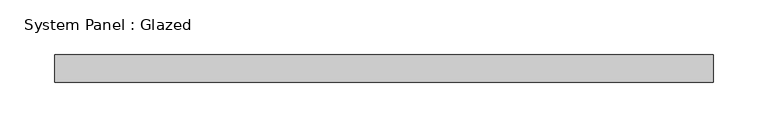
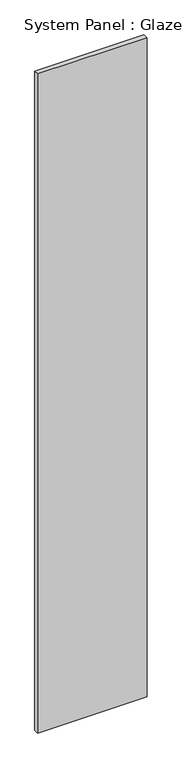
"""IFC4 building model written with IfcOpenShell, lengths in millimetres: plate geometry, System Panel : Glazed."""

from ifc_helpers import new_model, si_unit, origin, origin_with_axes, place, context, project, spatial, polyline, outline, extrude, source, transform, mapped, element, save


def system_panel_glazed_56e4e121(model_context):
    return source(origin(), model_context, "Body", "SweptSolid", [
        extrude(outline(polyline([(301.4636875, 19.05), (-301.4636875, 19.05), (-301.4636875, 44.45), (301.4636875, 44.45), (301.4636875, 19.05)])), origin_with_axes(), (0.0, 0.0, 1.0), 3835.4),
    ])


if __name__ == "__main__":
    model = new_model("IFC4")
    model_context = context("Model", 3, world=origin())
    ifc_project = project(units=[si_unit("LENGTHUNIT", "METRE", prefix="MILLI")], contexts=[model_context])
    site = spatial("IfcSite", under=ifc_project)
    building = spatial("IfcBuilding", under=site)
    placement = place(None, origin())
    system_panel_glazed_shape = system_panel_glazed_56e4e121(model_context)
    element("IfcPlate", 1, ObjectType="System Panel : Glazed", at=placement, inside=building, context=model_context, shape_type="MappedRepresentation", body=[
        mapped(system_panel_glazed_shape, transform((0.0, 0.0, 0.0), x_axis=(1.0, 0.0, 0.0), y_axis=(0.0, 1.0, 0.0), z_axis=(0.0, 0.0, 1.0))),
    ])
    save(model, "model.ifc")

# Revit data of these elements
# Type "System Panel : Glazed"
#   Construction Type Id = "GSP4R"
#   Analytic Construction = "1/8 in Pilkington single glazing"
#   Visual Light Transmittance = 0.9
#   Solar Heat Gain Coefficient = 0.86
#   Heat Transfer Coefficient (U) = 1.18115 BTU/(h·ft²·°F)
# Element 1 (IfcPlate, "System Panel : Glazed")
#   Materials on its faces: "Glass"
# Materials
#   "Glass": class "Glass", colour RGB 0 128 192, transparency 0.75, Description = "Soda Lime Glass", Cost = 0
